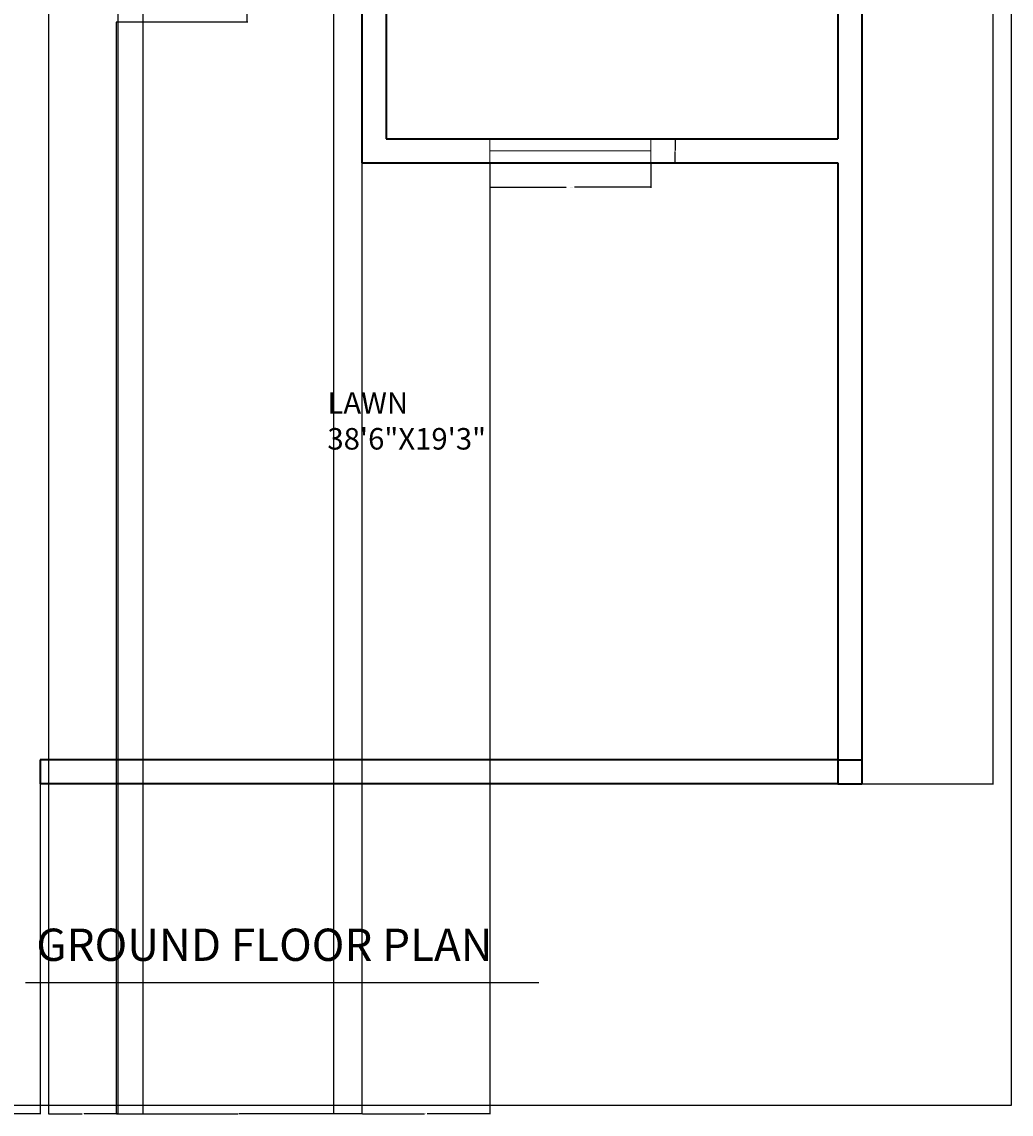
# Model space of a CAD drawing. Units: inches. Extents: x 2460 to 3031, y 933 to 2010.
# Tile 4 of 7: x 2663 to 3031, y 933 to 1339. Entities that reach past the tile are written whole.
import ezdxf

# ---------------------------------------------------------------- set-up
doc = ezdxf.new("R2010")
doc.units = ezdxf.units.IN
for name, color, linetype, lineweight in [('A-ANNO-DIMS', 2, 'Continuous', 18), ('A-ANNO-TTLB', 7, 'Continuous', 25), ('A-AREA-IDEN', 7, 'Continuous', 18), ('A-GLAZ', 4, 'Continuous', 18), ('A-WALL', 7, 'Continuous', 35), ('C-PROP', 7, 'Continuous', 35)]:
    doc.layers.add(name, color=color, linetype=linetype, lineweight=lineweight)
doc.styles.get("Standard").update_dxf_attribs({"font": 'arial.ttf'})
doc.dimstyles.get("Standard").update_dxf_attribs({"dimtxt": 0.18, "dimasz": 0.18, "dimexe": 0.18, "dimexo": 0.0625, "dimgap": 0.09, "dimtad": 0, "dimtih": 1, "dimtoh": 1, "dimdec": 4, "dimzin": 0, "dimdsep": 46, "dimtxsty": 'Standard', "dimcen": 0.09, "dimadec": 0, "dimazin": 0, "dimtfac": 1, "dimtdec": 4, "dimtofl": 0, "dimtmove": 0, "dimatfit": 3, "dimfxl": 1, "dimtolj": 1, "dimtzin": 0, "dimarcsym": 0})

# ---------------------------------------------------------------- blocks, each defined once
blk = doc.blocks.new('WIN-60')
for p, q in [((0, 9), (0, 0)), ((60, 4.5), (60, 9)), ((60, 9), (60, 0)), ((0, 0), (0, 4.5)), ((0, 4.5), (60, 4.5))]:
    blk.add_line(p, q)
blk = doc.blocks.new('*D30')
at = {"layer": 'A-ANNO-DIMS', "color": 0, "lineweight": -2, "transparency": 16777216}
for p, q in [((2836.67, 1286.92), (2836.67, 1277.8)), ((2896.67, 1286.92), (2896.67, 1277.8)), ((2836.85, 1277.98), (2865.1, 1277.98)), ((2896.49, 1277.98), (2868.25, 1277.98))]:
    blk.add_line(p, q, dxfattribs=at)
at = {"layer": 'A-ANNO-DIMS', "color": 0, "transparency": 16777216}
for points in [[(2836.85, 1278.01), (2836.85, 1277.95), (2836.67, 1277.98)], [(2896.49, 1278.01), (2896.49, 1277.95), (2896.67, 1277.98)]]:
    blk.add_solid(points, dxfattribs=at)
at = {"layer": 'Defpoints', "color": 0, "transparency": 16777216}
for p in [(2836.67, 1286.98), (2896.67, 1286.98), (2896.67, 1277.98)]:
    blk.add_point(p, dxfattribs=at)
at = {"layer": 'A-ANNO-DIMS', "color": 0, "transparency": 16777216, "insert": (2866.67, 1277.98), "char_height": 0.18, "attachment_point": 5}
blk.add_mtext('\\A1;FRONT WINDOW 60 TYP.', dxfattribs=at)
blk = doc.blocks.new('*D31')
at = {"layer": 'A-ANNO-DIMS', "color": 0, "lineweight": -2, "transparency": 16777216}
for p, q in [((2896.74, 1295.98), (2905.85, 1295.98)), ((2905.67, 1295.8), (2905.67, 1291.66)), ((2905.67, 1287.16), (2905.67, 1291.3)), ((2896.74, 1286.98), (2905.85, 1286.98))]:
    blk.add_line(p, q, dxfattribs=at)
at = {"layer": 'A-ANNO-DIMS', "color": 0, "transparency": 16777216}
for points in [[(2905.64, 1295.8), (2905.7, 1295.8), (2905.67, 1295.98)], [(2905.64, 1287.16), (2905.7, 1287.16), (2905.67, 1286.98)]]:
    blk.add_solid(points, dxfattribs=at)
at = {"layer": 'Defpoints', "color": 0, "transparency": 16777216}
for p in [(2896.67, 1295.98), (2905.67, 1295.98), (2896.67, 1286.98)]:
    blk.add_point(p, dxfattribs=at)
at = {"layer": 'A-ANNO-DIMS', "color": 0, "transparency": 16777216, "insert": (2905.67, 1291.48), "char_height": 0.18, "attachment_point": 5}
blk.add_mtext('\\A1;9 TYP.', dxfattribs=at)
blk = doc.blocks.new('*D33')
at = {"layer": 'A-ANNO-DIMS', "color": 0, "lineweight": -2, "transparency": 16777216}
for p, q in [((2975.23, 1957.98), (3024.15, 1957.98)), ((3023.97, 1957.8), (3023.97, 1507.16)), ((3023.97, 1056.16), (3023.97, 1506.8)), ((2975.23, 1055.98), (3024.15, 1055.98))]:
    blk.add_line(p, q, dxfattribs=at)
at = {"layer": 'A-ANNO-DIMS', "color": 0, "transparency": 16777216}
for points in [[(3023.94, 1957.8), (3024, 1957.8), (3023.97, 1957.98)], [(3023.94, 1056.16), (3024, 1056.16), (3023.97, 1055.98)]]:
    blk.add_solid(points, dxfattribs=at)
at = {"layer": 'Defpoints', "color": 0, "transparency": 16777216}
for p in [(2975.17, 1957.98), (3023.97, 1957.98), (2975.17, 1055.98)]:
    blk.add_point(p, dxfattribs=at)
at = {"layer": 'A-ANNO-DIMS', "color": 0, "transparency": 16777216, "insert": (3023.97, 1506.98), "char_height": 0.18, "attachment_point": 5}
blk.add_mtext('\\A1;902', dxfattribs=at)
blk = doc.blocks.new('*D34')
at = {"layer": 'A-ANNO-DIMS', "color": 0, "lineweight": -2, "transparency": 16777216}
for p, q in [((2520.67, 1055.92), (2520.67, 933.16)), ((2669.43, 1055.92), (2669.43, 933.16)), ((2520.85, 933.34), (2594.6, 933.34)), ((2669.25, 933.34), (2595.51, 933.34))]:
    blk.add_line(p, q, dxfattribs=at)
at = {"layer": 'A-ANNO-DIMS', "color": 0, "transparency": 16777216}
for points in [[(2520.85, 933.37), (2520.85, 933.31), (2520.67, 933.34)], [(2669.25, 933.37), (2669.25, 933.31), (2669.43, 933.34)]]:
    blk.add_solid(points, dxfattribs=at)
at = {"layer": 'Defpoints', "color": 0, "transparency": 16777216}
for p in [(2520.67, 1055.98), (2669.43, 1055.98), (2669.43, 933.34)]:
    blk.add_point(p, dxfattribs=at)
at = {"layer": 'A-ANNO-DIMS', "color": 0, "transparency": 16777216, "insert": (2595.05, 933.34), "char_height": 0.18, "attachment_point": 5}
blk.add_mtext('\\A1;148.76', dxfattribs=at)
blk = doc.blocks.new('*D36')
at = {"layer": 'A-ANNO-DIMS', "color": 0, "lineweight": -2, "transparency": 16777216}
for p, q in [((2697.67, 1339.42), (2697.67, 933.16)), ((2789.17, 1286.92), (2789.17, 933.16)), ((2697.85, 933.34), (2743.09, 933.34)), ((2788.99, 933.34), (2743.74, 933.34))]:
    blk.add_line(p, q, dxfattribs=at)
at = {"layer": 'A-ANNO-DIMS', "color": 0, "transparency": 16777216}
for points in [[(2697.85, 933.37), (2697.85, 933.31), (2697.67, 933.34)], [(2788.99, 933.37), (2788.99, 933.31), (2789.17, 933.34)]]:
    blk.add_solid(points, dxfattribs=at)
at = {"layer": 'Defpoints', "color": 0, "transparency": 16777216}
for p in [(2697.67, 1339.48), (2789.17, 1286.98), (2789.17, 933.34)]:
    blk.add_point(p, dxfattribs=at)
at = {"layer": 'A-ANNO-DIMS', "color": 0, "transparency": 16777216, "insert": (2743.42, 933.34), "char_height": 0.18, "attachment_point": 5}
blk.add_mtext('\\A1;91.5', dxfattribs=at)
blk = doc.blocks.new('*D38')
at = {"layer": 'A-ANNO-DIMS', "color": 0, "lineweight": -2, "transparency": 16777216}
for p, q in [((2672.51, 1591.25), (2672.51, 933.16)), ((2698.37, 1591.25), (2698.37, 933.16)), ((2672.69, 933.34), (2685.04, 933.34)), ((2698.19, 933.34), (2685.83, 933.34))]:
    blk.add_line(p, q, dxfattribs=at)
at = {"layer": 'A-ANNO-DIMS', "color": 0, "transparency": 16777216}
for points in [[(2672.69, 933.37), (2672.69, 933.31), (2672.51, 933.34)], [(2698.19, 933.37), (2698.19, 933.31), (2698.37, 933.34)]]:
    blk.add_solid(points, dxfattribs=at)
at = {"layer": 'Defpoints', "color": 0, "transparency": 16777216}
for p in [(2672.51, 1591.31), (2698.37, 1591.31), (2698.37, 933.34)]:
    blk.add_point(p, dxfattribs=at)
at = {"layer": 'A-ANNO-DIMS', "color": 0, "transparency": 16777216, "insert": (2685.44, 933.34), "char_height": 0.18, "attachment_point": 5}
blk.add_mtext('\\A1;25.87', dxfattribs=at)
blk = doc.blocks.new('*D43')
at = {"layer": 'A-ANNO-DIMS', "color": 0, "lineweight": -2, "transparency": 16777216}
for p, q in [((2707.62, 1374.89), (2707.62, 933.16)), ((2778.55, 1374.89), (2778.55, 933.16)), ((2707.8, 933.34), (2742.69, 933.34)), ((2778.37, 933.34), (2743.48, 933.34))]:
    blk.add_line(p, q, dxfattribs=at)
at = {"layer": 'A-ANNO-DIMS', "color": 0, "transparency": 16777216}
for points in [[(2707.8, 933.37), (2707.8, 933.31), (2707.62, 933.34)], [(2778.37, 933.37), (2778.37, 933.31), (2778.55, 933.34)]]:
    blk.add_solid(points, dxfattribs=at)
at = {"layer": 'Defpoints', "color": 0, "transparency": 16777216}
for p in [(2707.62, 1374.95), (2778.55, 1374.95), (2778.55, 933.34)]:
    blk.add_point(p, dxfattribs=at)
at = {"layer": 'A-ANNO-DIMS', "color": 0, "transparency": 16777216, "insert": (2743.09, 933.34), "char_height": 0.18, "attachment_point": 5}
blk.add_mtext('\\A1;70.93', dxfattribs=at)
blk = doc.blocks.new('*D45')
at = {"layer": 'A-ANNO-DIMS', "color": 0, "lineweight": -2, "transparency": 16777216}
for p, q in [((2789.17, 1286.92), (2789.17, 933.16)), ((2836.67, 1286.92), (2836.67, 933.16)), ((2789.35, 933.34), (2812.45, 933.34)), ((2836.49, 933.34), (2813.39, 933.34))]:
    blk.add_line(p, q, dxfattribs=at)
at = {"layer": 'A-ANNO-DIMS', "color": 0, "transparency": 16777216}
for points in [[(2789.35, 933.37), (2789.35, 933.31), (2789.17, 933.34)], [(2836.49, 933.37), (2836.49, 933.31), (2836.67, 933.34)]]:
    blk.add_solid(points, dxfattribs=at)
at = {"layer": 'Defpoints', "color": 0, "transparency": 16777216}
for p in [(2789.17, 1286.98), (2836.67, 1286.98), (2836.67, 933.34)]:
    blk.add_point(p, dxfattribs=at)
at = {"layer": 'A-ANNO-DIMS', "color": 0, "transparency": 16777216, "insert": (2812.92, 933.34), "char_height": 0.18, "attachment_point": 5}
blk.add_mtext('\\A1;47.505', dxfattribs=at)
blk = doc.blocks.new('*D51')
at = {"layer": 'A-ANNO-DIMS', "color": 0, "lineweight": -2, "transparency": 16777216}
for p, q in [((2697.73, 1374.95), (2746.65, 1374.95)), ((2746.47, 1374.77), (2746.47, 1357.4)), ((2746.47, 1339.66), (2746.47, 1357.03)), ((2697.73, 1339.48), (2746.65, 1339.48))]:
    blk.add_line(p, q, dxfattribs=at)
at = {"layer": 'A-ANNO-DIMS', "color": 0, "transparency": 16777216}
for points in [[(2746.44, 1374.77), (2746.5, 1374.77), (2746.47, 1374.95)], [(2746.44, 1339.66), (2746.5, 1339.66), (2746.47, 1339.48)]]:
    blk.add_solid(points, dxfattribs=at)
at = {"layer": 'Defpoints', "color": 0, "transparency": 16777216}
for p in [(2697.67, 1374.95), (2697.67, 1339.48), (2746.47, 1339.48)]:
    blk.add_point(p, dxfattribs=at)
at = {"layer": 'A-ANNO-DIMS', "color": 0, "transparency": 16777216, "insert": (2746.47, 1357.22), "char_height": 0.18, "attachment_point": 5}
blk.add_mtext('\\A1;35.466', dxfattribs=at)

msp = doc.modelspace()

# ---------------------------------------------------------------- linework, layer by layer
at = {"layer": 'A-ANNO-TTLB'}
msp.add_line((2664.0373, 982.1406), (2854.9139, 982.1406), dxfattribs=at)
msp.add_lwpolyline([(2459.8083, 2009.7942), (3030.6598, 2009.7942), (3030.6598, 936.3732), (2459.8083, 936.3732)], close=True, dxfattribs=at)
at = {"layer": 'A-WALL'}
for p, q in [((2966.1684, 1495.4828), (2966.1684, 1295.9828)), ((2798.1684, 1450.7932), (2798.1684, 1295.9828)), ((2789.1684, 1449.0529), (2789.1684, 1286.9828)), ((2798.1684, 1295.9828), (2966.1684, 1295.9828)), ((2894.1684, 1295.9828), (2966.1684, 1295.9828)), ((2789.1684, 1286.9828), (2966.1684, 1286.9828))]:
    msp.add_line(p, q, dxfattribs=at)
at = {"layer": 'C-PROP'}
for p, q in [((2975.1684, 1957.9828), (2975.1684, 1055.9828)), ((2966.1684, 1286.9828), (2966.1684, 1055.9828)), ((2966.1684, 1286.9828), (2966.1684, 1055.9828)), ((2966.1684, 1064.9828), (2669.433, 1064.9828)), ((2669.433, 1064.9828), (2669.433, 1055.9828)), ((2966.1684, 1064.9828), (2975.1684, 1064.9828)), ((2966.1684, 1055.9828), (2669.433, 1055.9828)), ((2966.1684, 1055.9828), (2975.1684, 1055.9828))]:
    msp.add_line(p, q, dxfattribs=at)

# ---------------------------------------------------------------- block references
at = {"layer": 'A-GLAZ'}
msp.add_blockref('WIN-60', (2836.673, 1286.983), dxfattribs=at)

# ---------------------------------------------------------------- texts
at = {"layer": 'A-ANNO-TTLB', "insert": (2668.0206, 1002.1717), "char_height": 12, "attachment_point": 1}
msp.add_mtext_dynamic_manual_height_columns('GROUND FLOOR PLAN', width=342.433643, gutter_width=12.5, heights=[0], dxfattribs=at)
at = {"layer": 'A-AREA-IDEN', "insert": (2776.2992, 1201.7157), "char_height": 8, "attachment_point": 1}
msp.add_mtext_dynamic_manual_height_columns('LAWN\\P38\'6"X19\'3"', width=189.86926, gutter_width=12.5, heights=[0], dxfattribs=at)

# ---------------------------------------------------------------- dimensions: what is measured, and where the dimension line sits
at = {"layer": 'A-ANNO-DIMS'}
for base, p1, p2, angle, override, picture, middle in [((3023.9679, 1957.9828), (2975.1684, 1055.9828), (2975.1684, 1957.9828), 90, {"dimdec": 0, "dimlfac": 1, "dimrnd": 0, "dimzin": 0, "dimdsep": 46, "dimlunit": 2}, '*D33', (3023.9679, 1506.9828)), ((2746.4679, 1339.4828), (2697.6684, 1374.9491), (2697.6684, 1339.4828), 270, {"dimdec": 3, "dimlfac": 1, "dimrnd": 0, "dimzin": 0, "dimdsep": 46, "dimlunit": 2}, '*D51', (2746.4679, 1357.216))]:
    dim = msp.add_linear_dim(base=base, p1=p1, p2=p2, angle=angle, dimstyle='Standard', override=override, dxfattribs=at)
    dim.commit()
    dim.dimension.update_dxf_attribs({"geometry": picture, "text_midpoint": middle})
for base, p1, p2, override, picture, middle in [((2698.3735, 933.3411), (2672.5051, 1591.3081), (2698.3735, 1591.3082), {"dimdec": 2, "dimlfac": 1, "dimrnd": 0, "dimzin": 0, "dimdsep": 46, "dimlunit": 2}, '*D38', (2685.4393, 933.3411)), ((2778.5542, 933.3411), (2707.6216, 1374.9491), (2778.5542, 1374.9491), {"dimdec": 2, "dimlfac": 1, "dimrnd": 0, "dimzin": 0, "dimdsep": 46, "dimlunit": 2}, '*D43', (2743.0879, 933.3411)), ((2789.1684, 933.3411), (2697.6684, 1339.4828), (2789.1684, 1286.9828), {"dimdec": 1, "dimlfac": 1, "dimrnd": 0, "dimzin": 0, "dimdsep": 46, "dimlunit": 2}, '*D36', (2743.4184, 933.3411)), ((2836.6734, 933.3411), (2789.1684, 1286.9828), (2836.6734, 1286.9828), {"dimdec": 3, "dimlfac": 1, "dimrnd": 0, "dimzin": 0, "dimdsep": 46, "dimlunit": 2}, '*D45', (2812.9209, 933.3411)), ((2669.433, 933.3411), (2520.6684, 1055.9828), (2669.433, 1055.9828), {"dimdec": 2, "dimlfac": 1, "dimrnd": 0, "dimzin": 0, "dimdsep": 46, "dimlunit": 2}, '*D34', (2595.0507, 933.3411))]:
    dim = msp.add_linear_dim(base=base, p1=p1, p2=p2, dimstyle='Standard', override=override, dxfattribs=at)
    dim.commit()
    dim.dimension.update_dxf_attribs({"geometry": picture, "text_midpoint": middle})
dim = msp.add_linear_dim(base=(2905.6734, 1295.9828), p1=(2896.6734, 1286.9828), p2=(2896.6734, 1295.9828), angle=90, text='<> TYP.', dimstyle='Standard', override={"dimdec": 0, "dimlfac": 1, "dimrnd": 0, "dimzin": 0, "dimdsep": 46, "dimlunit": 2}, dxfattribs=at)
dim.commit()
dim.dimension.update_dxf_attribs({"geometry": '*D31', "text_midpoint": (2905.6734, 1291.4828)})
dim = msp.add_linear_dim(base=(2896.6734, 1277.9828), p1=(2836.6734, 1286.9828), p2=(2896.6734, 1286.9828), text='FRONT WINDOW <> TYP.', dimstyle='Standard', override={"dimdec": 0, "dimlfac": 1, "dimrnd": 0, "dimzin": 0, "dimdsep": 46, "dimlunit": 2}, dxfattribs=at)
dim.commit()
dim.dimension.update_dxf_attribs({"geometry": '*D30', "text_midpoint": (2866.6734, 1277.9828)})

doc.saveas('drawing.dxf')
